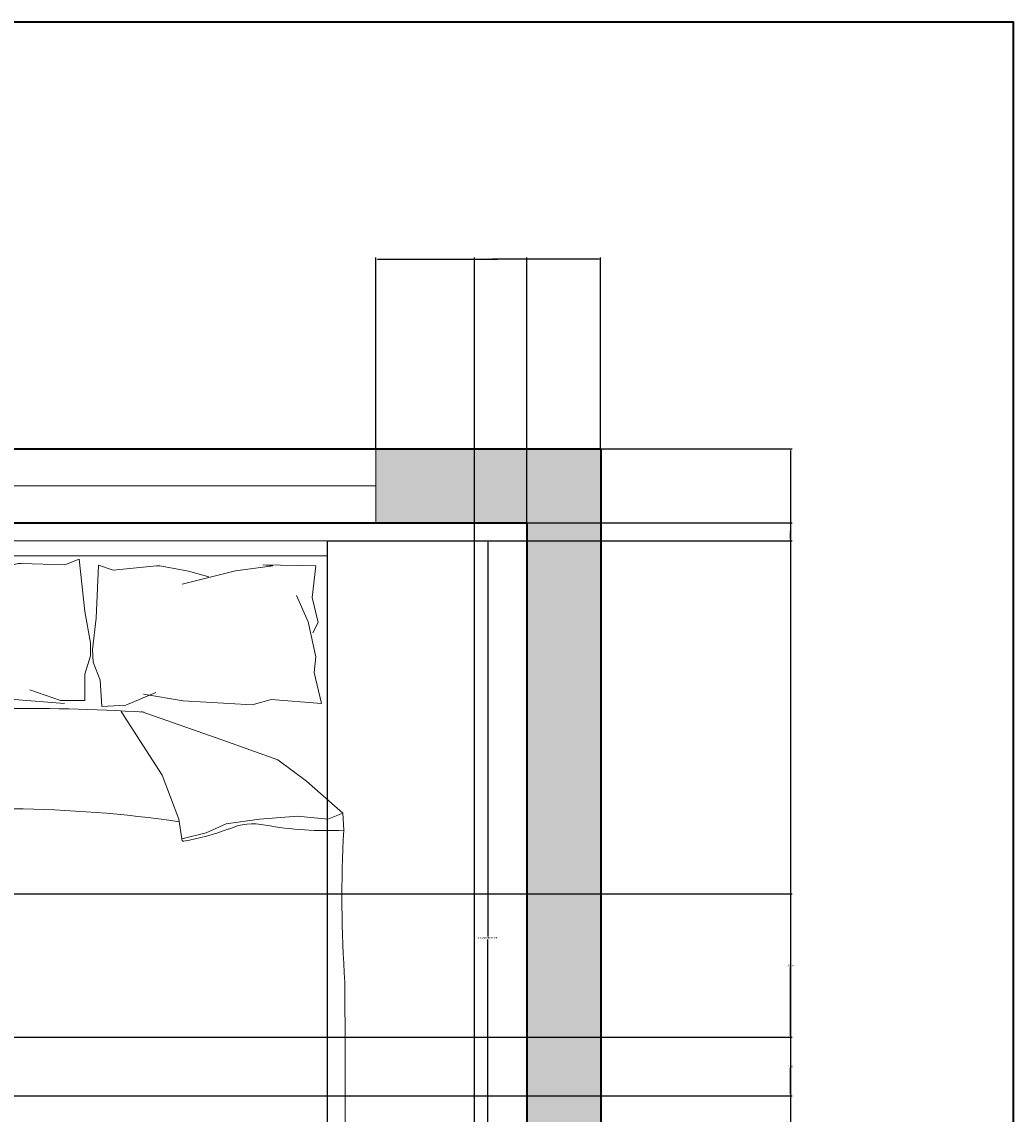
# Model space of a CAD drawing. Units: inches. Extents: x 2606 to 3027, y 1906 to 2463.
# Tile 10 of 10: x 2906 to 3027, y 2329 to 2463. Entities that reach past the tile are written whole.
import ezdxf

# ---------------------------------------------------------------- set-up
doc = ezdxf.new("R2010")
doc.units = ezdxf.units.IN
for name, color, linetype, lineweight in [('A-ANNO-DIMS', 2, 'Continuous', 18), ('A-ANNO-TTLB', 7, 'Continuous', 35), ('A-FURN', 8, 'Continuous', 13), ('A-GLAZ', 4, 'Continuous', 18), ('A-WALL', 7, 'Continuous', 35)]:
    doc.layers.add(name, color=color, linetype=linetype, lineweight=lineweight)
doc.layers.add('A-WALL-PATT', color=251, linetype='Continuous', lineweight=13, true_color=0x636466)
doc.styles.get("Standard").update_dxf_attribs({"font": 'arial.ttf'})
doc.dimstyles.get("Standard").update_dxf_attribs({"dimtxt": 0.18, "dimasz": 0.18, "dimexe": 0.18, "dimexo": 0.0625, "dimgap": 0.09, "dimtad": 0, "dimtih": 1, "dimtoh": 1, "dimdec": 4, "dimzin": 0, "dimdsep": 46, "dimtxsty": 'Standard', "dimcen": 0.09, "dimadec": 0, "dimazin": 0, "dimtfac": 1, "dimtdec": 4, "dimtofl": 0, "dimtmove": 0, "dimatfit": 3, "dimfxl": 1, "dimtolj": 1, "dimtzin": 0, "dimarcsym": 0})

# ---------------------------------------------------------------- blocks, each defined once
blk = doc.blocks.new('BED-DOUBLE')
for p, q in [((4.17, 75.16), (4.17, 96.87)), ((4.17, 96.87), (61.46, 96.87)), ((61.46, 96.87), (61.46, 64.97)), ((4.17, 95.03), (61.46, 95.03)), ((20.24, 93.24), (23.7, 94.11)), ((23.7, 94.11), (24.09, 94.11)), ((24.09, 94.11), (29.42, 93.94)), ((29.42, 93.94), (31.15, 94.63)), ((31.15, 94.63), (31.84, 88.22)), ((33.54, 93.89), (33.25, 87.44)), ((35.31, 93.3), (33.54, 93.89)), ((40.62, 93.81), (35.31, 93.3)), ((41.01, 93.83), (40.62, 93.81)), ((44.52, 93.18), (41.01, 93.83)), ((54.8, 93.82), (50.25, 93.19)), ((60.08, 93.81), (53.6, 93.92)), ((53.6, 93.92), (54.8, 93.82)), ((60.08, 93.81), (59.62, 89.96)), ((4.67, 92.87), (9.81, 93.27)), ((4.67, 92.9), (5.36, 89.08)), ((9.81, 93.27), (9.93, 93.24)), ((9.93, 93.24), (14.52, 92.9)), ((14.52, 92.9), (21.1, 91.68)), ((17.81, 92.38), (20.24, 93.24)), ((50.25, 93.19), (43.75, 91.57)), ((47, 92.47), (44.52, 93.18)), ((6.06, 86.14), (7.27, 89.43)), ((59.12, 86.97), (57.7, 90.18)), ((59.62, 89.96), (60.34, 86.88)), ((5.36, 89.08), (4.84, 85.96)), ((31.84, 88.22), (32.54, 84.4)), ((33.25, 87.44), (32.79, 83.59)), ((60.08, 82.69), (59.12, 86.97)), ((60.34, 86.88), (59.72, 85.62)), ((4.84, 85.96), (5.54, 84.75)), ((5.36, 81.8), (6.06, 86.14)), ((32.54, 84.4), (32.54, 82.84)), ((32.54, 82.84), (31.84, 80.59)), ((32.79, 83.59), (32.89, 82.03)), ((5.71, 79.9), (5.36, 81.8)), ((32.89, 82.03), (33.72, 79.83)), ((59.85, 80.77), (60.08, 82.69)), ((31.84, 80.59), (31.84, 77.38)), ((60.78, 77), (59.85, 80.77)), ((5.02, 76.08), (5.71, 79.9)), ((33.72, 79.83), (33.92, 76.62)), ((7.65, 78.14), (12.48, 77.34)), ((20.89, 76.82), (23.24, 77.49)), ((23.24, 77.49), (29.39, 77)), ((28.9, 77.38), (25.13, 78.68)), ((36.87, 76.8), (40.55, 78.34)), ((39.04, 78.14), (43.87, 77.34)), ((52.28, 76.82), (54.63, 77.49)), ((54.63, 77.49), (60.78, 77)), ((11.13, 76.95), (5.02, 76.08)), ((12.48, 77.34), (11.13, 76.95)), ((12.48, 77.34), (20.89, 76.82)), ((31.84, 77.38), (28.9, 77.38)), ((33.92, 76.62), (36.87, 76.8)), ((43.87, 77.34), (52.28, 76.82)), ((36.28, 76.03), (41.3, 68.25)), ((48.73, 72.52), (38.73, 76.03)), ((55.41, 70.1), (48.73, 72.52)), ((58.94, 67.51), (55.41, 70.1)), ((41.3, 68.25), (43.34, 62.87)), ((63.38, 63.61), (58.94, 67.51)), ((43.34, 62.87), (43.71, 60.45)), ((49.1, 62.31), (53.18, 62.87)), ((53.18, 62.87), (57.82, 63.24)), ((57.82, 63.24), (61.54, 62.87)), ((61.54, 62.87), (63.38, 63.61)), ((63.48, 61.52), (63.38, 63.61, 4.64)), ((46.68, 61.2), (49.1, 62.31)), ((43.71, 60.45), (46.68, 61.2)), ((18.06, 1.87), (47.57, 1.87))]:
    blk.add_line(p, q)
for centre, radius, start, end in [((25.61, -121.38), 197.77, 86.0865, 96.7821), ((102.1, 72.78), 99.87, 178.7218, 185.604), ((21.29, -90.53), 154.68, 81.7845, 96.9006), ((-200.58, 59.5), 203.94, 358.4762, 1.0082), ((37.35, 95.1), 35.55, 280.6617, 289.8806), ((52.44, 54.83), 7.46, 78.6608, 113.7384), ((61.53, 104.85), 43.38, 259.8763, 272.5657), ((218.51, 53.34), 155.25, 176.9791, 183.8365), ((43.92, 60.38), 0.221, 160.2464, 271.1377), ((581.23, 36.19), 578.22, 178.22771, 181.71854), ((-5405.34, 15.56), 5469.02, 0.00217, 0.28689), ((-32.25, 19.53), 35.53, 346.0648, 358.9113), ((91.3, 14.55), 27.65, 177.4714, 206.4681), ((-25.97, 12.62), 28.25, 337.9751, 356.652), ((-20.65, 125.3), 127.63, 283.3832, 287.7053), ((1.3, 1.3), 1.31, 146.1736, 293.4781), ((25.69, -143.9), 145.97, 92.9958, 99.4091), ((49.34, -157.62), 159.5, 84.4998, 90.6351), ((65.23, 2.32), 1.32, 242.6588, 356.02)]:
    blk.add_arc(centre, radius, start, end)
blk = doc.blocks.new('WIN-60IN')
for p, q in [((0, 9), (0, 0)), ((60, 4.5), (60, 9)), ((60, 9), (60, 0)), ((0, 0), (0, 4.5)), ((0, 4.5), (60, 4.5))]:
    blk.add_line(p, q)
blk = doc.blocks.new('*D9')
at = {"layer": 'A-ANNO-DIMS', "color": 0, "lineweight": -2, "transparency": 16777216}
for p, q in [((2948.82, 2399.4), (2963.48, 2399.4)), ((2963.3, 2399.22), (2963.3, 2351.08)), ((2963.3, 2302.58), (2963.3, 2350.71)), ((2948.82, 2302.4), (2963.48, 2302.4))]:
    blk.add_line(p, q, dxfattribs=at)
at = {"layer": 'A-ANNO-DIMS', "color": 0, "transparency": 16777216}
for points in [[(2963.27, 2399.22), (2963.33, 2399.22), (2963.3, 2399.4)], [(2963.27, 2302.58), (2963.33, 2302.58), (2963.3, 2302.4)]]:
    blk.add_solid(points, dxfattribs=at)
at = {"layer": 'Defpoints', "color": 0, "transparency": 16777216}
for p in [(2948.75, 2399.4), (2963.3, 2399.4), (2948.75, 2302.4)]:
    blk.add_point(p, dxfattribs=at)
at = {"layer": 'A-ANNO-DIMS', "color": 0, "transparency": 16777216, "insert": (2963.3, 2350.9), "char_height": 0.18, "attachment_point": 5}
blk.add_mtext('\\A1;DOUBLE BED 97 TYP.', dxfattribs=at)
blk = doc.blocks.new('*D26')
at = {"layer": 'A-ANNO-DIMS', "color": 0, "lineweight": -2, "transparency": 16777216}
for p, q in [((2977.13, 2410.61), (3000.44, 2410.61)), ((3000.26, 2410.43), (3000.26, 2199.79)), ((3000.26, 1988.79), (3000.26, 2199.43)), ((2977.13, 1988.61), (3000.44, 1988.61))]:
    blk.add_line(p, q, dxfattribs=at)
at = {"layer": 'A-ANNO-DIMS', "color": 0, "transparency": 16777216}
for points in [[(3000.23, 2410.43), (3000.29, 2410.43), (3000.26, 2410.61)], [(3000.23, 1988.79), (3000.29, 1988.79), (3000.26, 1988.61)]]:
    blk.add_solid(points, dxfattribs=at)
at = {"layer": 'Defpoints', "color": 0, "transparency": 16777216}
for p in [(2977.06, 2410.61), (3000.26, 2410.61), (2977.06, 1988.61)]:
    blk.add_point(p, dxfattribs=at)
at = {"layer": 'A-ANNO-DIMS', "color": 0, "transparency": 16777216, "insert": (3000.26, 2199.61), "char_height": 0.18, "attachment_point": 5}
blk.add_mtext('\\A1;422', dxfattribs=at)
blk = doc.blocks.new('*D30')
at = {"layer": 'A-ANNO-DIMS', "color": 0, "lineweight": -2, "transparency": 16777216}
for p, q in [((2949.62, 2410.67), (2949.62, 2433.99)), ((2949.8, 2433.81), (2962.87, 2433.81)), ((2976.88, 2433.81), (2963.81, 2433.81)), ((2977.06, 2410.67), (2977.06, 2433.99))]:
    blk.add_line(p, q, dxfattribs=at)
at = {"layer": 'A-ANNO-DIMS', "color": 0, "transparency": 16777216}
for points in [[(2949.8, 2433.84), (2949.8, 2433.78), (2949.62, 2433.81)], [(2976.88, 2433.84), (2976.88, 2433.78), (2977.06, 2433.81)]]:
    blk.add_solid(points, dxfattribs=at)
at = {"layer": 'Defpoints', "color": 0, "transparency": 16777216}
for p in [(2977.06, 2433.81), (2949.62, 2410.61), (2977.06, 2410.61)]:
    blk.add_point(p, dxfattribs=at)
at = {"layer": 'A-ANNO-DIMS', "color": 0, "transparency": 16777216, "insert": (2963.34, 2433.81), "char_height": 0.18, "attachment_point": 5}
blk.add_mtext('\\A1;27.445', dxfattribs=at)
blk = doc.blocks.new('*D49')
at = {"layer": 'A-ANNO-DIMS', "color": 0, "lineweight": -2, "transparency": 16777216}
for p, q in [((2847.63, 2356.26), (3000.44, 2356.26)), ((3000.26, 2356.08), (3000.26, 2347.69)), ((3000.26, 2338.93), (3000.26, 2347.32)), ((2847.63, 2338.75), (3000.44, 2338.75))]:
    blk.add_line(p, q, dxfattribs=at)
at = {"layer": 'A-ANNO-DIMS', "color": 0, "transparency": 16777216}
for points in [[(3000.23, 2356.08), (3000.29, 2356.08), (3000.26, 2356.26)], [(3000.23, 2338.93), (3000.29, 2338.93), (3000.26, 2338.75)]]:
    blk.add_solid(points, dxfattribs=at)
at = {"layer": 'Defpoints', "color": 0, "transparency": 16777216}
for p in [(2847.56, 2356.26), (3000.26, 2356.26), (2847.56, 2338.75)]:
    blk.add_point(p, dxfattribs=at)
at = {"layer": 'A-ANNO-DIMS', "color": 0, "transparency": 16777216, "insert": (3000.26, 2347.51), "char_height": 0.18, "attachment_point": 5}
blk.add_mtext('\\A1;17.516', dxfattribs=at)
blk = doc.blocks.new('*D53')
at = {"layer": 'A-ANNO-DIMS', "color": 0, "lineweight": -2, "transparency": 16777216}
for p, q in [((2847.63, 2338.75), (3000.44, 2338.75)), ((3000.26, 2338.57), (3000.26, 2335.36)), ((3000.26, 2331.79), (3000.26, 2335)), ((2847.63, 2331.61), (3000.44, 2331.61))]:
    blk.add_line(p, q, dxfattribs=at)
at = {"layer": 'A-ANNO-DIMS', "color": 0, "transparency": 16777216}
for points in [[(3000.23, 2338.57), (3000.29, 2338.57), (3000.26, 2338.75)], [(3000.23, 2331.79), (3000.29, 2331.79), (3000.26, 2331.61)]]:
    blk.add_solid(points, dxfattribs=at)
at = {"layer": 'Defpoints', "color": 0, "transparency": 16777216}
for p in [(2847.56, 2338.75), (3000.26, 2338.75), (2847.56, 2331.61)]:
    blk.add_point(p, dxfattribs=at)
at = {"layer": 'A-ANNO-DIMS', "color": 0, "transparency": 16777216, "insert": (3000.26, 2335.18), "char_height": 0.18, "attachment_point": 5}
blk.add_mtext('\\A1;7.138', dxfattribs=at)
blk = doc.blocks.new('*D75')
at = {"layer": 'A-ANNO-DIMS', "color": 0, "lineweight": -2, "transparency": 16777216}
for p, q in [((2968.06, 2401.55), (2968.06, 1965.23)), ((2943.67, 2399.33), (2943.67, 1965.23)), ((2943.85, 1965.41), (2955.4, 1965.41)), ((2967.88, 1965.41), (2956.33, 1965.41))]:
    blk.add_line(p, q, dxfattribs=at)
at = {"layer": 'A-ANNO-DIMS', "color": 0, "transparency": 16777216}
for points in [[(2943.85, 1965.44), (2943.85, 1965.38), (2943.67, 1965.41)], [(2967.88, 1965.44), (2967.88, 1965.38), (2968.06, 1965.41)]]:
    blk.add_solid(points, dxfattribs=at)
at = {"layer": 'Defpoints', "color": 0, "transparency": 16777216}
for p in [(2968.06, 2401.61), (2943.67, 2399.4), (2968.06, 1965.41)]:
    blk.add_point(p, dxfattribs=at)
at = {"layer": 'A-ANNO-DIMS', "color": 0, "transparency": 16777216, "insert": (2955.86, 1965.41), "char_height": 0.18, "attachment_point": 5}
blk.add_mtext('\\A1;24.397', dxfattribs=at)
blk = doc.blocks.new('*D77')
at = {"layer": 'A-ANNO-DIMS', "color": 0, "lineweight": -2, "transparency": 16777216}
for p, q in [((2961.66, 2034.29), (2961.66, 2433.99)), ((2961.84, 2433.81), (2964.47, 2433.81)), ((2967.88, 2433.81), (2965.26, 2433.81)), ((2968.06, 2032.67), (2968.06, 2433.99))]:
    blk.add_line(p, q, dxfattribs=at)
at = {"layer": 'A-ANNO-DIMS', "color": 0, "transparency": 16777216}
for points in [[(2961.84, 2433.84), (2961.84, 2433.78), (2961.66, 2433.81)], [(2967.88, 2433.84), (2967.88, 2433.78), (2968.06, 2433.81)]]:
    blk.add_solid(points, dxfattribs=at)
at = {"layer": 'Defpoints', "color": 0, "transparency": 16777216}
for p in [(2968.06, 2433.81), (2961.66, 2034.23), (2968.06, 2032.61)]:
    blk.add_point(p, dxfattribs=at)
at = {"layer": 'A-ANNO-DIMS', "color": 0, "transparency": 16777216, "insert": (2964.86, 2433.81), "char_height": 0.18, "attachment_point": 5}
blk.add_mtext('\\A1;6.402', dxfattribs=at)
blk = doc.blocks.new('*D79')
at = {"layer": 'A-ANNO-DIMS', "color": 0, "lineweight": -2, "transparency": 16777216}
for p, q in [((2949.68, 2401.61), (3000.44, 2401.61)), ((3000.26, 2401.43), (3000.26, 2400.68)), ((2943.73, 2399.4), (3000.44, 2399.4)), ((3000.26, 2399.58), (3000.26, 2400.32))]:
    blk.add_line(p, q, dxfattribs=at)
at = {"layer": 'A-ANNO-DIMS', "color": 0, "transparency": 16777216}
for points in [[(3000.23, 2401.43), (3000.29, 2401.43), (3000.26, 2401.61)], [(3000.23, 2399.58), (3000.29, 2399.58), (3000.26, 2399.4)]]:
    blk.add_solid(points, dxfattribs=at)
at = {"layer": 'Defpoints', "color": 0, "transparency": 16777216}
for p in [(2949.62, 2401.61), (3000.26, 2401.61), (2943.67, 2399.4)]:
    blk.add_point(p, dxfattribs=at)
at = {"layer": 'A-ANNO-DIMS', "color": 0, "transparency": 16777216, "insert": (3000.26, 2400.5), "char_height": 0.18, "attachment_point": 5}
blk.add_mtext('\\A1;2.21', dxfattribs=at)

msp = doc.modelspace()

# ---------------------------------------------------------------- hatches: boundary and pattern name
at = {"layer": 'A-WALL-PATT'}
h = msp.add_hatch(color=256, dxfattribs=at)
h.dxf.hatch_style = 1
h.paths.add_polyline_path([(2667.063, 2401.6097), (2691.9697, 2401.6097), (2691.9697, 2406.1097), (2691.9697, 2410.6097), (2658.063, 2410.6097), (2658.063, 2238.7051), (2667.063, 2238.7051)])
h.paths.add_polyline_path([(2804.9965, 2406.1097), (2804.9965, 2410.6097), (2751.9697, 2410.6097), (2751.9697, 2401.6097), (2783.063, 2401.6097), (2783.063, 2257.6097), (2778.6739, 2257.6097), (2778.6739, 2253.1097), (2792.3386, 2253.1097), (2792.3386, 2255.3597), (2792.3386, 2257.6097), (2787.563, 2257.6097), (2787.563, 2327.1097), (2847.563, 2327.1097), (2847.563, 2331.6097), (2787.563, 2331.6097), (2787.563, 2401.6097), (2804.9965, 2401.6097)])
h.paths.add_polyline_path([(2889.6183, 2406.1097), (2889.6183, 2410.6097), (2828.9965, 2410.6097), (2828.9965, 2401.6097), (2831.8174, 2401.6097), (2847.563, 2401.6097), (2847.563, 2357.8311), (2849.813, 2357.8311), (2852.063, 2357.8311), (2852.063, 2401.6097), (2889.6183, 2401.6097)])
h.paths.add_polyline_path([(2977.063, 2410.6097), (2949.6183, 2410.6097), (2949.6183, 2401.6097), (2968.063, 2401.6097), (2968.063, 2157.1097), (2897.063, 2157.1097), (2897.063, 2174.1966), (2892.563, 2174.1966), (2892.563, 2157.1097), (2886.8122, 2157.1097), (2886.8122, 2152.6097), (2968.063, 2152.6097), (2968.063, 2032.6097), (2950.8911, 2032.6097), (2950.8911, 2028.1097), (2968.063, 2028.1097), (2968.063, 1993.1097), (2852.063, 1993.1097), (2852.063, 2028.1097), (2856.0743, 2028.1097), (2856.0743, 2030.3597), (2856.0743, 2032.6097), (2852.063, 2032.6097), (2852.063, 2152.6097), (2857.369, 2152.6097), (2857.369, 2154.8597), (2857.369, 2157.1097), (2847.563, 2157.1097), (2847.563, 2152.6097), (2847.563, 1993.1097), (2837.0415, 1993.1097), (2837.0415, 1988.6097), (2977.063, 1988.6097)])
h.paths.add_polyline_path([(2968.063, 2257.6097), (2886.9679, 2257.6097), (2886.9679, 2253.1097), (2892.563, 2253.1097), (2892.563, 2215.1332), (2897.063, 2215.1332), (2897.063, 2253.1097), (2968.063, 2253.1097)], flags=17)
h.paths.add_polyline_path([(2856.057, 2255.3597), (2856.057, 2257.6097), (2852.063, 2257.6097), (2852.063, 2336.7476), (2849.813, 2336.7476), (2847.563, 2336.7476), (2847.563, 2331.6097), (2847.563, 2327.1097), (2847.563, 2257.6097), (2813.482, 2257.6097), (2813.482, 2253.1097), (2856.057, 2253.1097)])
h.paths.add_polyline_path([(2748.8874, 2255.3597), (2748.8874, 2257.6097), (2667.063, 2257.6097), (2667.063, 2253.1097), (2748.8874, 2253.1097)])
h.paths.add_polyline_path([(2667.063, 2152.6097), (2744.8238, 2152.6097), (2744.8238, 2154.8597), (2744.8238, 2157.1097), (2667.063, 2157.1097), (2667.063, 2178.7051), (2658.063, 2178.7051), (2658.063, 1988.6097), (2801.0415, 1988.6097), (2801.0415, 1990.8597), (2801.0415, 1993.1097), (2787.563, 1993.1097), (2787.563, 2157.1097), (2777.1295, 2157.1097), (2777.1295, 2152.6097), (2783.063, 2152.6097), (2783.063, 2032.6097), (2778.4484, 2032.6097), (2778.4484, 2028.1097), (2783.063, 2028.1097), (2783.063, 1993.1097), (2667.063, 1993.1097), (2667.063, 2028.1097), (2680.1652, 2028.1097), (2680.1652, 2030.3597), (2680.1652, 2032.6097), (2667.063, 2032.6097)])
h.paths.add_polyline_path([(2755.4074, 2032.6097), (2728.1652, 2032.6097), (2728.1652, 2028.1097), (2755.4074, 2028.1097), (2755.4074, 2030.3597)], flags=17)
h.paths.add_polyline_path([(2902.8911, 2030.3597), (2902.8911, 2032.6097), (2877.6885, 2032.6097), (2877.6885, 2028.1097), (2902.8911, 2028.1097)], flags=17)
h.paths.add_polyline_path([(2810.2211, 2267.221), (2851.2716, 2267.221), (2851.2716, 2289.6098), (2810.2211, 2289.6098)], flags=9)

# ---------------------------------------------------------------- linework, layer by layer
at = {"layer": 'A-ANNO-TTLB'}
msp.add_lwpolyline([(2605.9227, 2462.7868), (3027.4339, 2462.7868), (3027.4339, 1905.5336), (2605.9227, 1905.5336)], close=True, dxfattribs=at)
at = {"layer": 'A-WALL'}
for p, q in [((2658.063, 2410.6097), (2977.063, 2410.6097)), ((2977.063, 2410.6097), (2977.063, 1988.6097)), ((2852.063, 2401.6097), (2968.063, 2401.6097)), ((2968.063, 2401.6097), (2968.063, 2157.1097))]:
    msp.add_line(p, q, dxfattribs=at)

# ---------------------------------------------------------------- block references
at = {"layer": 'A-FURN'}
msp.add_blockref('BED-DOUBLE', (2882.206, 2302.524), dxfattribs=at)
at = {"layer": 'A-GLAZ'}
msp.add_blockref('WIN-60IN', (2889.6187, 2401.61), dxfattribs=at)

# ---------------------------------------------------------------- dimensions: what is measured, and where the dimension line sits
at = {"layer": 'A-ANNO-DIMS'}
for base, p1, p2, picture, middle in [((2977.063, 2433.8097), (2949.6183, 2410.6097), (2977.063, 2410.6097), '*D30', (2963.3407, 2433.8097)), ((2968.063, 2433.8097), (2961.6611, 2034.2301), (2968.063, 2032.6097), '*D77', (2964.8621, 2433.8097)), ((2968.063, 1965.4097), (2943.6661, 2399.3963), (2968.063, 2401.6097), '*D75', (2955.8645, 1965.4097))]:
    dim = msp.add_linear_dim(base=base, p1=p1, p2=p2, dimstyle='Standard', override={"dimdec": 3, "dimlfac": 1, "dimrnd": 0, "dimzin": 0, "dimdsep": 46, "dimlunit": 2}, dxfattribs=at)
    dim.commit()
    dim.dimension.update_dxf_attribs({"geometry": picture, "text_midpoint": middle})
for base, p1, p2, override, picture, middle in [((3000.263, 2410.6097), (2977.063, 1988.6097), (2977.063, 2410.6097), {"dimdec": 0, "dimlfac": 1, "dimrnd": 0, "dimzin": 0, "dimdsep": 46, "dimlunit": 2}, '*D26', (3000.263, 2199.6097)), ((3000.263, 2401.6097), (2943.6661, 2399.3963), (2949.6183, 2401.6097), {"dimdec": 2, "dimlfac": 1, "dimrnd": 0, "dimzin": 0, "dimdsep": 46, "dimlunit": 2}, '*D79', (3000.263, 2400.503)), ((3000.263, 2356.2638), (2847.563, 2338.7476), (2847.563, 2356.2638), {"dimdec": 3, "dimlfac": 1, "dimrnd": 0, "dimzin": 0, "dimdsep": 46, "dimlunit": 2}, '*D49', (3000.263, 2347.5057)), ((3000.263, 2338.7476), (2847.563, 2331.6097), (2847.563, 2338.7476), {"dimdec": 3, "dimlfac": 1, "dimrnd": 0, "dimzin": 0, "dimdsep": 46, "dimlunit": 2}, '*D53', (3000.263, 2335.1787))]:
    dim = msp.add_linear_dim(base=base, p1=p1, p2=p2, angle=90, dimstyle='Standard', override=override, dxfattribs=at)
    dim.commit()
    dim.dimension.update_dxf_attribs({"geometry": picture, "text_midpoint": middle})
dim = msp.add_linear_dim(base=(2963.3041, 2399.3963), p1=(2948.7543, 2302.3976), p2=(2948.7543, 2399.3963), angle=90, text='DOUBLE BED <> TYP.', dimstyle='Standard', override={"dimdec": 0, "dimlfac": 1, "dimrnd": 0, "dimzin": 0, "dimdsep": 46, "dimlunit": 2}, dxfattribs=at)
dim.commit()
dim.dimension.update_dxf_attribs({"geometry": '*D9', "text_midpoint": (2963.3041, 2350.897)})

doc.saveas('drawing.dxf')
